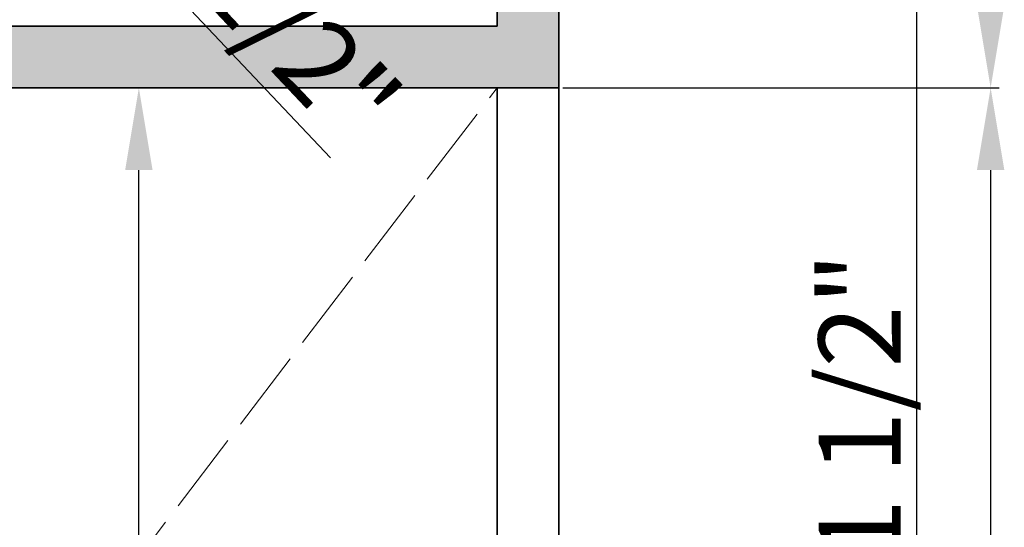
# Model space of a CAD drawing. Units: inches. Extents: x 2083 to 3317, y 1141 to 2115.
# Tile 254 of 256: x 3048 to 3192, y 1639 to 1713. Entities that reach past the tile are written whole.
import ezdxf

# ---------------------------------------------------------------- set-up
doc = ezdxf.new("R2010")
doc.units = ezdxf.units.IN
doc.linetypes.add('ACAD_ISO02W100', pattern=[15, 12, -3])
for name, color, linetype, lineweight in [('A-ANNO-DIMS', 2, 'Continuous', 18), ('A-FLOR-OPEN', 8, 'ACAD_ISO02W100', 13), ('A-WALL', 7, 'Continuous', 35)]:
    doc.layers.add(name, color=color, linetype=linetype, lineweight=lineweight)
doc.layers.add('A-WALL-PATT', color=251, linetype='Continuous', lineweight=13, true_color=0x636466)
doc.styles.get("Standard").update_dxf_attribs({"font": 'arial.ttf'})
doc.dimstyles.new('ISO-25', dxfattribs={"dimtxt": 12, "dimasz": 12, "dimexe": 1.25, "dimexo": 0.625, "dimtad": 1, "dimlunit": 3, "dimtxsty": 'Standard', "dimcen": 2.5, "dimadec": 0, "dimazin": 0, "dimtfac": 1, "dimtmove": 0, "dimatfit": 3, "dimfxl": 1, "dimarcsym": 0})

# ---------------------------------------------------------------- blocks, each defined once
blk = doc.blocks.new('*D7')
at = {"layer": 'A-ANNO-DIMS', "color": 0, "lineweight": -2, "transparency": 16777216}
for p, q in [((3127.58, 2020.76), (3191.32, 2020.76)), ((3190.07, 2008.76), (3190.07, 1714.76)), ((3127.58, 1702.76), (3191.32, 1702.76))]:
    blk.add_line(p, q, dxfattribs=at)
at = {"layer": 'A-ANNO-DIMS', "color": 0, "transparency": 16777216}
for points in [[(3188.07, 2008.76), (3192.07, 2008.76), (3190.07, 2020.76)], [(3188.07, 1714.76), (3192.07, 1714.76), (3190.07, 1702.76)]]:
    blk.add_solid(points, dxfattribs=at)
at = {"layer": 'Defpoints', "color": 0, "transparency": 16777216}
for p in [(3126.96, 2020.76), (3126.96, 1702.76), (3190.07, 1702.76)]:
    blk.add_point(p, dxfattribs=at)
at = {"layer": 'A-ANNO-DIMS', "color": 0, "transparency": 16777216, "insert": (3183.32, 1861.76), "char_height": 12, "attachment_point": 5, "rotation": 90}
blk.add_mtext('26\'-6"', dxfattribs=at)
blk = doc.blocks.new('*D8')
at = {"layer": 'A-ANNO-DIMS', "color": 0, "lineweight": -2, "transparency": 16777216}
for p, q in [((3127.58, 1702.76), (3191.32, 1702.76)), ((3190.07, 1690.76), (3190.07, 1498.76)), ((3127.58, 1486.76), (3191.32, 1486.76))]:
    blk.add_line(p, q, dxfattribs=at)
at = {"layer": 'A-ANNO-DIMS', "color": 0, "transparency": 16777216}
for points in [[(3188.07, 1690.76), (3192.07, 1690.76), (3190.07, 1702.76)], [(3188.07, 1498.76), (3192.07, 1498.76), (3190.07, 1486.76)]]:
    blk.add_solid(points, dxfattribs=at)
at = {"layer": 'Defpoints', "color": 0, "transparency": 16777216}
for p in [(3126.96, 1702.76), (3126.96, 1486.76), (3190.07, 1486.76)]:
    blk.add_point(p, dxfattribs=at)
at = {"layer": 'A-ANNO-DIMS', "color": 0, "transparency": 16777216, "insert": (3183.32, 1594.76), "char_height": 12, "attachment_point": 5, "rotation": 90}
blk.add_mtext("18'", dxfattribs=at)
blk = doc.blocks.new('*D35')
at = {"layer": 'A-ANNO-DIMS', "color": 0, "lineweight": -2, "transparency": 16777216}
for p, q in [((3127.58, 2020.76), (3180.56, 2020.76)), ((3179.31, 1275.26), (3179.31, 2008.76)), ((3127.58, 1263.26), (3180.56, 1263.26))]:
    blk.add_line(p, q, dxfattribs=at)
at = {"layer": 'A-ANNO-DIMS', "color": 0, "transparency": 16777216}
for points in [[(3177.31, 2008.76), (3181.31, 2008.76), (3179.31, 2020.76)], [(3177.31, 1275.26), (3181.31, 1275.26), (3179.31, 1263.26)]]:
    blk.add_solid(points, dxfattribs=at)
at = {"layer": 'Defpoints', "color": 0, "transparency": 16777216}
for p in [(3126.96, 2020.76), (3179.31, 2020.76), (3126.96, 1263.26)]:
    blk.add_point(p, dxfattribs=at)
at = {"layer": 'A-ANNO-DIMS', "color": 0, "transparency": 16777216, "insert": (3172.48, 1642.01), "char_height": 12, "attachment_point": 5, "rotation": 90}
blk.add_mtext('63\'-1 1/2"', dxfattribs=at)
blk = doc.blocks.new('*D65')
at = {"layer": 'A-ANNO-DIMS', "color": 0, "lineweight": -2, "transparency": 16777216}
for p, q in [((3117.33, 1702.76), (3064.36, 1702.76)), ((3065.61, 1498.76), (3065.61, 1690.76)), ((3117.33, 1486.76), (3064.36, 1486.76))]:
    blk.add_line(p, q, dxfattribs=at)
at = {"layer": 'A-ANNO-DIMS', "color": 0, "transparency": 16777216}
for points in [[(3063.61, 1690.76), (3067.61, 1690.76), (3065.61, 1702.76)], [(3063.61, 1498.76), (3067.61, 1498.76), (3065.61, 1486.76)]]:
    blk.add_solid(points, dxfattribs=at)
at = {"layer": 'Defpoints', "color": 0, "transparency": 16777216}
for p in [(3065.61, 1702.76), (3117.96, 1702.76), (3117.96, 1486.76)]:
    blk.add_point(p, dxfattribs=at)
at = {"layer": 'A-ANNO-DIMS', "color": 0, "transparency": 16777216, "insert": (3058.86, 1594.76), "char_height": 12, "attachment_point": 5, "rotation": 90}
blk.add_mtext('18\'-0"', dxfattribs=at)
blk = doc.blocks.new('*D71')
at = {"layer": 'A-ANNO-DIMS', "color": 0, "lineweight": -2, "transparency": 16777216}
for p, q in [((2997.14, 1794.66), (3020.88, 1769.53)), ((3093.61, 1692.52), (3029.12, 1760.8))]:
    blk.add_line(p, q, dxfattribs=at)
at = {"layer": 'A-ANNO-DIMS', "color": 0, "transparency": 16777216}
blk.add_solid([(3030.57, 1762.18), (3027.67, 1759.43), (3020.88, 1769.53)], dxfattribs=at)
at = {"layer": 'Defpoints', "color": 0, "transparency": 16777216}
for p in [(2997.14, 1794.66), (3020.88, 1769.53)]:
    blk.add_point(p, dxfattribs=at)
at = {"layer": 'A-ANNO-DIMS', "color": 0, "transparency": 16777216, "insert": (3070.45, 1726.99), "char_height": 12, "attachment_point": 5, "rotation": 313.3638}
blk.add_mtext('R2\'-10 1/2"', dxfattribs=at)

msp = doc.modelspace()

# ---------------------------------------------------------------- hatches: boundary and pattern name
at = {"layer": 'A-WALL-PATT'}
h = msp.add_hatch(color=256, dxfattribs=at)
h.dxf.hatch_style = 1
h.paths.add_polyline_path([(3126.96, 2020.761), (2748.96, 2020.761), (2604.96, 2020.761), (2226.96, 2020.761), (2226.96, 1702.761), (2466.96, 1702.761), (2466.96, 1582.761), (2418.96, 1582.761), (2418.96, 1477.761), (2226.96, 1477.761), (2226.96, 1263.261), (2544.96, 1263.261), (2544.96, 1411.761), (2604.96, 1411.761), (2685.96, 1411.761), (2685.96, 1420.761), (2604.96, 1420.761), (2604.96, 1573.761), (2604.96, 1702.761), (2604.96, 2011.761), (2748.96, 2011.761), (2748.96, 1702.761), (2862.96, 1702.761), (2862.96, 1621.761), (2871.96, 1621.761), (2871.96, 1702.761), (2883.96, 1702.761), (2883.96, 1706.939, -0.0264593), (2883.96, 1711.761), (2757.96, 1711.761), (2757.96, 1807.761), (2787.96, 1807.761), (2787.96, 1812.261), (2757.96, 1812.261), (2757.96, 2011.761), (2877.96, 2011.761), (2877.96, 1812.261), (2847.96, 1812.261), (2847.96, 1807.761), (2889.836, 1807.761), (2889.836, 1812.261), (2882.46, 1812.261), (2882.46, 2011.761), (3117.96, 2011.761), (3117.96, 1812.261), (2937.836, 1812.261), (2937.836, 1807.761), (2995.71, 1807.761), (2995.71, 1796.118), (3000.21, 1796.118), (3000.21, 1807.761), (3117.96, 1807.761), (3117.96, 1711.761), (3000.21, 1711.761), (3000.21, 1760.118), (2998.573, 1760.118, -0.020711), (2995.71, 1760.118), (2995.71, 1711.761), (2931.96, 1711.761), (2931.96, 1702.761), (3126.96, 1702.761)])
h.paths.add_polyline_path([(2471.46, 2011.761), (2471.46, 1810.011), (2462.717, 1810.011), (2462.717, 1805.511), (2505.96, 1805.511), (2505.96, 1810.011), (2475.96, 1810.011), (2475.96, 2011.761), (2595.96, 2011.761), (2595.96, 1810.011), (2565.96, 1810.011), (2565.96, 1805.511), (2595.96, 1805.511), (2595.96, 1711.761), (2235.96, 1711.761), (2235.96, 1805.511), (2353.71, 1805.511), (2353.71, 1796.054), (2358.21, 1796.054), (2358.21, 1805.511), (2414.717, 1805.511), (2414.717, 1810.011), (2235.96, 1810.011), (2235.96, 2011.761)], flags=16)
h.paths.add_polyline_path([(2270.205, 1994.61), (2270.205, 1970.61), (2246.205, 1970.61), (2246.205, 1994.61)], flags=0)
edge = h.paths.add_edge_path(flags=0)
edge.add_ellipse((2332.027, 1899.798), major_axis=(-3.043, 3.043), ratio=0.1682525, start_angle=-161.33217, end_angle=-156.30711, ccw=False)
edge.add_ellipse((2333.082, 1898.744), major_axis=(-1.055, 1.055), ratio=0.4535321, start_angle=-123.37102, end_angle=-94.15911)
edge = h.paths.add_edge_path(flags=0)
edge.add_ellipse((2332.027, 1968.876), major_axis=(3.043, 3.043), ratio=0.1682525, start_angle=18.66783, end_angle=23.69289)
edge.add_spline(control_points=[(2332.926, 1970.691), (2332.227, 1970.336), (2330.894, 1969.659), (2328.413, 1970.932), (2327.204, 1967.749), (2324.71, 1969.956), (2322.533, 1967.012), (2320.013, 1971.296), (2317.68, 1968.158), (2316.041, 1967.102), (2315.427, 1966.81)], knot_values=[0, 0, 0, 0, 2.2670587, 4.3245589, 6.6855835, 8.8786411, 11.121502, 14.300359, 17.7552837, 19.732645, 19.732645, 19.732645, 19.732645], degree=3, periodic=0)
edge.add_ellipse((2332.027, 1968.876), major_axis=(3.043, 3.043), ratio=0.1682525, start_angle=18.66783, end_angle=23.69289, ccw=False)
edge.add_ellipse((2333.082, 1969.931), major_axis=(1.055, 1.055), ratio=0.4535321, start_angle=56.62898, end_angle=85.84089, ccw=False)
edge = h.paths.add_edge_path(flags=0)
edge.add_spline(control_points=[(2296.428, 1967.988), (2293.628, 1965.336), (2287.704, 1959.727), (2299.744, 1949.996), (2294.533, 1935.669), (2290.573, 1920.604), (2293.394, 1909.974), (2296.185, 1904.967)], knot_values=[0.0991853, 0.0991853, 0.0991853, 0.0991853, 0.3453009, 0.6198217, 0.9826526, 1.3860932, 1.8105546, 1.8105546, 1.8105546, 1.8105546], degree=3, periodic=0)
edge.add_spline(control_points=[(2296.185, 1904.967), (2297.384, 1902.619), (2298.001, 1901.949), (2298.553, 1901.468)], knot_values=[0.0062457, 0.0062457, 0.0062457, 0.0062457, 0.0554759, 0.0554759, 0.0554759, 0.0554759], degree=3, periodic=0)
edge.add_spline(control_points=[(2298.553, 1901.468), (2297.259, 1900.923), (2295.225, 1900.232), (2293.06, 1900.614), (2292.101, 1900.788), (2292.09, 1900.791)], knot_values=[0.3128349, 0.3128349, 0.3128349, 0.3128349, 0.4017797, 0.4749867, 0.4759027, 0.4759027, 0.4759027, 0.4759027], degree=3, periodic=0)
edge.add_arc((2292.794, 1904.664), 3.937, 215.4209, 259.69818, ccw=False)
edge.add_spline(control_points=[(2289.585, 1902.382), (2289.477, 1902.535), (2289.368, 1902.688), (2289.261, 1902.841)], knot_values=[0.1028719, 0.1028719, 0.1028719, 0.1028719, 0.1168958, 0.1168958, 0.1168958, 0.1168958], degree=3, periodic=0)
edge.add_spline(control_points=[(2289.261, 1902.841), (2288.687, 1902.55), (2287.64, 1902.02), (2285.881, 1901.874), (2283.853, 1901.504), (2281.72, 1899.711), (2278.467, 1899.493), (2276.157, 1901.883), (2272.259, 1899.804), (2267.778, 1901.843), (2262.244, 1900.184), (2257.415, 1901.782), (2254.318, 1900.726), (2253.178, 1900.337)], knot_values=[0, 0, 0, 0, 1.9079767, 3.4771759, 5.261074, 7.9728515, 11.6802485, 13.7179214, 16.9395917, 22.789562, 27.5025027, 33.5952153, 37.1456181, 37.1456181, 37.1456181, 37.1456181], degree=3, periodic=0)
edge.add_line((2253.178, 1900.337), (2250.244, 1902.841))
edge.add_line((2250.244, 1902.841), (2250.244, 1965.833))
edge.add_line((2250.244, 1965.833), (2253.178, 1968.337))
edge.add_spline(control_points=[(2253.178, 1968.337), (2254.318, 1967.948), (2257.415, 1966.892), (2262.244, 1968.49), (2267.778, 1966.831), (2271.527, 1968.537), (2273.876, 1967.828), (2274.207, 1967.728)], knot_values=[0, 0, 0, 0, 0.0901802, 0.2449351, 0.3646438, 0.5132331, 0.5378548, 0.5378548, 0.5378548, 0.5378548], degree=3, periodic=0)
edge.add_arc((2274.353, 1963.793), 3.937, 72.05113, 92.12795, ccw=False)
edge.add_arc((2281.297, 1985.23), 18.596, 252.05113, 288.56572)
edge.add_arc((2292.317, 1956.029), 12.646, 71.02679, 113.77822, ccw=False)
edge = h.paths.add_edge_path(flags=0)
edge.add_spline(control_points=[(2274.899, 1951.856), (2275.066, 1951.617), (2275.233, 1951.377), (2275.398, 1951.136)], knot_values=[1.4099157, 1.4099157, 1.4099157, 1.4099157, 1.4315903, 1.4315903, 1.4315903, 1.4315903], degree=3, periodic=0)
edge.add_spline(control_points=[(2275.398, 1951.136), (2275.792, 1950.562), (2276.179, 1949.984), (2276.546, 1949.397)], knot_values=[1.3582378, 1.3582378, 1.3582378, 1.3582378, 1.4099157, 1.4099157, 1.4099157, 1.4099157], degree=3, periodic=0)
edge.add_line((2276.546, 1949.397), (2277.437, 1947.862))
edge.add_spline(control_points=[(2277.437, 1947.862), (2276.304, 1945.673), (2274.64, 1942.427), (2274.632, 1938.094), (2272.799, 1930.852), (2274.356, 1943.897), (2275.948, 1947.923), (2276.546, 1949.397)], knot_values=[0.0056315, 0.0056315, 0.0056315, 0.0056315, 0.1860139, 0.2660015, 0.3570872, 0.5963902, 0.7397317, 0.7397317, 0.7397317, 0.7397317], degree=3, periodic=0)
edge.add_spline(control_points=[(2276.546, 1949.397), (2276.179, 1949.984), (2275.792, 1950.562), (2275.398, 1951.136)], knot_values=[1.3582378, 1.3582378, 1.3582378, 1.3582378, 1.4099157, 1.4099157, 1.4099157, 1.4099157], degree=3, periodic=0)
edge.add_spline(control_points=[(2275.398, 1951.136), (2274.943, 1950.08), (2274.208, 1948.025), (2273.935, 1944.851), (2272.469, 1937.627), (2273.466, 1945.696), (2274.701, 1951.059), (2274.899, 1951.856)], knot_values=[0.1043639, 0.1043639, 0.1043639, 0.1043639, 0.1896363, 0.2696239, 0.3607096, 0.6000126, 0.6446217, 0.6446217, 0.6446217, 0.6446217], degree=3, periodic=0)
h.paths.add_polyline_path([(2269.168, 1963.128, -0.3575267), (2268.171, 1960.976, -0.0925607), (2268.171, 1939.436, -0.3575267), (2269.168, 1937.285, -0.3575267), (2267.016, 1938.282, -0.1647847), (2254.686, 1938.282, -0.3575267), (2252.534, 1937.285, -0.3575267), (2253.531, 1939.436, -0.0925607), (2253.531, 1960.976, -0.3575267), (2252.534, 1963.128, -0.3575267), (2254.686, 1962.131, -0.1647847), (2267.016, 1962.131, -0.3575267)], flags=0)
h.paths.add_polyline_path([(2248.874, 1967.802), (2248.874, 1957.028), (2249.458, 1957.028), (2249.458, 1911.647), (2248.874, 1911.647), (2248.874, 1900.873), (2246.512, 1900.873, 0.1973271), (2244.15, 1902.457), (2244.15, 1966.218, 0.1973271), (2246.512, 1967.802)], flags=0)
h.paths.add_polyline_path([(2269.168, 1931.389, -0.3575267), (2268.171, 1929.238, -0.0925607), (2268.171, 1907.698, -0.3575267), (2269.168, 1905.547, -0.3575267), (2267.016, 1906.544, -0.1647847), (2254.686, 1906.544, -0.3575267), (2252.534, 1905.547, -0.3575267), (2253.531, 1907.698, -0.0925607), (2253.531, 1929.238, -0.3575267), (2252.534, 1931.389, -0.3575267), (2254.686, 1930.392, -0.1647847), (2267.016, 1930.392, -0.3575267)], flags=0)
edge = h.paths.add_edge_path(flags=0)
edge.add_spline(control_points=[(2276.197, 1906.724), (2276.168, 1909.029), (2276.114, 1913.372), (2270.598, 1924.925), (2273.905, 1919.013), (2275.922, 1916.262), (2275.475, 1912.402), (2277.258, 1910.381), (2276.696, 1908.225), (2276.646, 1906.813), (2276.618, 1906.008)], knot_values=[0, 0, 0, 0, 8.6102597, 16.2212739, 18.8430575, 23.8048978, 27.4408283, 29.3561016, 31.2034776, 33.6506866, 33.6506866, 33.6506866, 33.6506866], degree=3, periodic=0)
edge.add_spline(control_points=[(2276.618, 1906.008), (2276.623, 1905.624), (2276.498, 1904.629), (2275.442, 1903.855), (2274.937, 1903.08), (2274.859, 1902.841)], knot_values=[0.1564884, 0.1564884, 0.1564884, 0.1564884, 0.1843975, 0.2313765, 0.2505985, 0.2505985, 0.2505985, 0.2505985], degree=3, periodic=0)
edge.add_line((2274.859, 1902.841), (2276.506, 1902.841))
edge.add_spline(control_points=[(2276.506, 1902.841), (2276.788, 1903.085), (2277.665, 1904.125), (2278.25, 1904.341), (2277.654, 1908.527), (2278.156, 1906.228), (2278.1, 1905.286), (2278.847, 1904.069), (2277.857, 1903.415), (2277.874, 1902.991), (2277.904, 1902.841)], knot_values=[0.0595743, 0.0595743, 0.0595743, 0.0595743, 0.0807529, 0.1037415, 0.1697201, 0.1760361, 0.2071372, 0.2404744, 0.2623409, 0.2736605, 0.2736605, 0.2736605, 0.2736605], degree=3, periodic=0)
edge.add_line((2277.904, 1902.841), (2280.03, 1902.841))
edge.add_spline(control_points=[(2280.03, 1902.841), (2279.888, 1903.088), (2279.499, 1903.982), (2280.152, 1905.939), (2278.104, 1909.658), (2279.762, 1907.185), (2280.328, 1904.875), (2280.485, 1903.49), (2281.463, 1903.249), (2281.758, 1902.936), (2281.834, 1902.841)], knot_values=[0.013856, 0.013856, 0.013856, 0.013856, 0.0348738, 0.0888667, 0.1078792, 0.1267378, 0.158714, 0.1937575, 0.2174868, 0.2267221, 0.2267221, 0.2267221, 0.2267221], degree=3, periodic=0)
edge.add_spline(control_points=[(2281.834, 1902.841), (2281.788, 1902.827), (2281.647, 1902.783), (2281.396, 1902.859), (2281.088, 1902.985), (2280.721, 1903.061), (2280.333, 1903.026), (2280.125, 1902.899), (2280.03, 1902.841)], knot_values=[0, 0, 0, 0, 0.1441304, 0.435517, 0.7492759, 1.1530457, 1.5483707, 1.878348, 1.878348, 1.878348, 1.878348], degree=3, periodic=0)
edge.add_line((2280.03, 1902.841), (2277.904, 1902.841))
edge.add_spline(control_points=[(2277.904, 1902.841), (2277.893, 1902.796), (2277.865, 1902.68), (2277.607, 1902.687), (2277.274, 1902.801), (2276.838, 1902.62), (2276.584, 1902.789), (2276.506, 1902.841)], knot_values=[0, 0, 0, 0, 0.1271885, 0.3261988, 0.6280094, 1.2435704, 1.5153306, 1.5153306, 1.5153306, 1.5153306], degree=3, periodic=0)
edge.add_line((2276.506, 1902.841), (2274.859, 1902.841))
edge.add_spline(control_points=[(2274.859, 1902.841), (2274.814, 1902.899), (2274.725, 1903.013), (2274.493, 1903.119), (2274.244, 1902.961), (2273.937, 1903.185), (2273.614, 1902.983), (2273.408, 1902.883), (2273.322, 1902.841)], knot_values=[0, 0, 0, 0, 0.2184302, 0.4369566, 0.6879766, 0.9903786, 1.3983955, 1.6918498, 1.6918498, 1.6918498, 1.6918498], degree=3, periodic=0)
edge.add_spline(control_points=[(2273.322, 1902.841), (2273.617, 1903.446), (2274.274, 1904.538), (2276.027, 1904.574), (2276.207, 1906.584), (2276.197, 1906.724)], knot_values=[0.0122268, 0.0122268, 0.0122268, 0.0122268, 0.0594721, 0.1062177, 0.134458, 0.134458, 0.134458, 0.134458], degree=3, periodic=0)
h.paths.add_polyline_path([(2270.776, 1897.79), (2270.776, 1873.79), (2246.776, 1873.79), (2246.776, 1897.79)], flags=0)
h.paths.add_polyline_path([(2353.71, 1760.005), (2353.71, 1760.054), (2358.21, 1760.054, -0.033729)], flags=0)
h.paths.add_polyline_path([(2321.819, 1737.529), (2341.995, 1737.529, -0.4142136), (2343.203, 1736.321), (2343.203, 1721.021, -0.4142136), (2341.995, 1719.813), (2321.819, 1719.813, -0.4142136), (2320.611, 1721.021), (2320.611, 1736.321, -0.4142136)], flags=0)
h.paths.add_polyline_path([(2324.235, 1736.321), (2339.579, 1736.321, -0.4142136), (2341.995, 1733.905), (2341.995, 1725.45, -0.4142136), (2339.579, 1723.034), (2333.681, 1723.034), (2333.845, 1722.045, -0.8706461), (2335.425, 1721.826, -0.767327), (2333.923, 1721.423), (2331.291, 1721.423, -0.767327), (2329.788, 1721.826, -0.8706461), (2331.368, 1722.045), (2331.533, 1723.034), (2324.235, 1723.034, -0.4142136), (2321.819, 1725.45), (2321.819, 1733.905, -0.4142136)], flags=0)
h.paths.add_polyline_path([(2570.484, 1928.615), (2589.684, 1928.615), (2590.169, 1928.615), (2590.169, 1904.993), (2570.484, 1904.993)], flags=0)
h.paths.add_polyline_path([(2574.447, 1927.264, -1), (2572.829, 1927.264, -1)], flags=0)
h.paths.add_polyline_path([(2573.09, 1926.941), (2573.925, 1927.776), (2574.148, 1927.553), (2573.313, 1926.718)], flags=0)
h.paths.add_polyline_path([(2578.779, 1919.73, -1), (2571.592, 1919.73, -1)], flags=0)
h.paths.add_polyline_path([(2578.385, 1919.73, -1), (2571.985, 1919.73, -1)], flags=0)
h.paths.add_polyline_path([(2331.596, 1729.476, -1), (2333.618, 1729.476, -1)], flags=0)
h.paths.add_polyline_path([(2578.034, 1927.264, -1), (2576.416, 1927.264, -1)], flags=0)
h.paths.add_polyline_path([(2576.689, 1927.531), (2576.912, 1927.754), (2577.747, 1926.919), (2577.524, 1926.696)], flags=0)
h.paths.add_polyline_path([(2578.139, 1909.86, -1), (2572.232, 1909.86, -1)], flags=0)
h.paths.add_polyline_path([(2577.745, 1909.86, -1), (2572.625, 1909.86, -1)], flags=0)
h.paths.add_polyline_path([(2583.798, 1927.264, -1), (2582.179, 1927.264, -1)], flags=0)
h.paths.add_polyline_path([(2582.719, 1927.754), (2583.554, 1926.919), (2583.331, 1926.696), (2582.496, 1927.531)], flags=0)
h.paths.add_polyline_path([(2582.496, 1927.531), (2582.719, 1927.754), (2583.554, 1926.919), (2583.331, 1926.696)], flags=0)
h.paths.add_polyline_path([(2587.739, 1920.53, -1), (2581.832, 1920.53, -1)], flags=0)
h.paths.add_polyline_path([(2587.345, 1920.53, -1), (2582.225, 1920.53, -1)], flags=0)
h.paths.add_polyline_path([(2587.385, 1927.264, -1), (2585.766, 1927.264, -1)], flags=0)
h.paths.add_polyline_path([(2586.082, 1926.98), (2586.917, 1927.815), (2587.14, 1927.593), (2586.305, 1926.758)], flags=0)
h.paths.add_polyline_path([(2588.379, 1910.66, -1), (2581.192, 1910.66, -1)], flags=0)
h.paths.add_polyline_path([(2587.985, 1910.66, -1), (2581.585, 1910.66, -1)], flags=0)
h.paths.add_polyline_path([(2417.168, 1729.478), (2437.344, 1729.478, -0.4142136), (2438.552, 1728.27), (2438.552, 1712.969, -0.4142136), (2437.344, 1711.761), (2417.168, 1711.761, -0.4142136), (2415.96, 1712.969), (2415.96, 1728.27, -0.4142136)], flags=0)
h.paths.add_polyline_path([(2419.584, 1728.27), (2434.928, 1728.27, -0.4142136), (2437.344, 1725.854), (2437.344, 1717.398, -0.4142136), (2434.928, 1714.983), (2429.029, 1714.983), (2429.194, 1713.994, -0.8706461), (2430.774, 1713.775, -0.767327), (2429.271, 1713.372), (2426.64, 1713.372, -0.767327), (2425.137, 1713.775, -0.8706461), (2426.717, 1713.994), (2426.882, 1714.983), (2419.584, 1714.983, -0.4142136), (2417.168, 1717.398), (2417.168, 1725.854, -0.4142136)], flags=0)
h.paths.add_polyline_path([(2419.584, 1728.27), (2434.928, 1728.27, -0.4142136), (2437.344, 1725.854), (2437.344, 1717.398, -0.4142136), (2434.928, 1714.983), (2429.029, 1714.983), (2428.358, 1719.009), (2427.553, 1719.009), (2426.882, 1714.983), (2419.584, 1714.983, -0.4142136), (2417.168, 1717.398), (2417.168, 1725.854, -0.4142136)], flags=0)
h.paths.add_polyline_path([(2426.944, 1721.425, -1), (2428.967, 1721.425, -1)], flags=0)
h.paths.add_polyline_path([(2475.96, 1702.761), (2595.96, 1702.761), (2595.96, 1582.761), (2475.96, 1582.761)], flags=16)
h.paths.add_polyline_path([(2427.96, 1573.761), (2595.96, 1573.761), (2595.96, 1468.761), (2595.96, 1420.761), (2384.46, 1420.761), (2384.46, 1468.761), (2427.96, 1468.761)], flags=16)
h.paths.add_polyline_path([(2379.96, 1468.761), (2379.96, 1420.761), (2235.96, 1420.761), (2235.96, 1468.761)], flags=16)
h.paths.add_polyline_path([(2317.816, 1466.696), (2337.992, 1466.696, -0.4142136), (2339.2, 1465.488), (2339.2, 1450.187, -0.4142136), (2337.992, 1448.979), (2317.816, 1448.979, -0.4142136), (2316.608, 1450.187), (2316.608, 1465.488, -0.4142136)], flags=0)
h.paths.add_polyline_path([(2320.232, 1465.488), (2335.576, 1465.488, -0.4142136), (2337.992, 1463.072), (2337.992, 1454.616, -0.4142136), (2335.576, 1452.2), (2329.677, 1452.2), (2329.842, 1451.212, -0.8706461), (2331.422, 1450.992, -0.767327), (2329.92, 1450.59), (2327.288, 1450.59, -0.767327), (2325.785, 1450.992, -0.8706461), (2327.365, 1451.212), (2327.53, 1452.2), (2320.232, 1452.2, -0.4142136), (2317.816, 1454.616), (2317.816, 1463.072, -0.4142136)], flags=0)
h.paths.add_polyline_path([(2320.232, 1465.488), (2335.576, 1465.488, -0.4142136), (2337.992, 1463.072), (2337.992, 1454.616, -0.4142136), (2335.576, 1452.2), (2329.677, 1452.2), (2329.006, 1456.227), (2328.201, 1456.227), (2327.53, 1452.2), (2320.232, 1452.2, -0.4142136), (2317.816, 1454.616), (2317.816, 1463.072, -0.4142136)], flags=0)
h.paths.add_polyline_path([(2327.593, 1458.643, -1), (2329.615, 1458.643, -1)], flags=0)
h.paths.add_polyline_path([(2244.412, 1433.34), (2241.921, 1433.34, -0.4142136), (2240.018, 1435.244), (2240.018, 1440.953, -0.4142105), (2241.921, 1442.856), (2244.412, 1442.856, -1.9764724)], flags=0)
h.paths.add_polyline_path([(2245.357, 1434.398, -0.4142136), (2245.357, 1441.799, -2.1440985)], flags=0)
h.paths.add_polyline_path([(2535.96, 1416.261), (2535.96, 1272.261), (2235.96, 1272.261), (2235.96, 1416.261)], flags=16)
h.paths.add_polyline_path([(2260.12, 1384.293), (2260.12, 1362.039), (2237.865, 1362.039), (2237.865, 1384.293)], flags=0)
edge = h.paths.add_edge_path(flags=0)
edge.add_line((2318.252, 1362.093), (2318.146, 1362.001))
edge.add_ellipse((2317.445, 1360.431), major_axis=(2.822, 2.822), ratio=0.1682525, start_angle=18.66783, end_angle=20.94813, ccw=False)
edge.add_ellipse((2318.423, 1361.409), major_axis=(0.978, 0.978), ratio=0.4535321, start_angle=56.62898, end_angle=70.2262, ccw=False)
edge = h.paths.add_edge_path(flags=0)
edge.add_line((2319.107, 1295.571), (2319.015, 1295.677))
edge.add_ellipse((2317.445, 1296.378), major_axis=(-2.822, 2.822), ratio=0.1682525, start_angle=-161.33217, end_angle=-159.05187, ccw=False)
edge.add_ellipse((2318.423, 1295.4), major_axis=(-0.978, 0.978), ratio=0.4535321, start_angle=-123.37102, end_angle=-109.7738)
edge = h.paths.add_edge_path(flags=0)
edge.add_spline(control_points=[(2284.21, 1301.17), (2284.581, 1300.445), (2284.891, 1299.892), (2285.16, 1299.461)], knot_values=[0.0390658, 0.0390658, 0.0390658, 0.0390658, 0.0554759, 0.0554759, 0.0554759, 0.0554759], degree=3, periodic=0)
edge.add_line((2285.16, 1299.461), (2284.21, 1301.17))
edge = h.paths.add_edge_path(flags=0)
edge.add_line((2280.412, 1297.298), (2283.37, 1297.036))
edge.add_line((2283.37, 1297.036), (2286.406, 1297.926))
edge.add_spline(control_points=[(2286.406, 1297.926), (2285.305, 1297.463), (2284.345, 1297.129), (2283.37, 1297.036)], knot_values=[0.3943688, 0.3943688, 0.3943688, 0.3943688, 0.4759027, 0.4759027, 0.4759027, 0.4759027], degree=3, periodic=0)
edge.add_spline(control_points=[(2283.37, 1297.036), (2283.281, 1297.028), (2282.316, 1296.957), (2281.313, 1297.134), (2280.423, 1297.296), (2280.412, 1297.298)], knot_values=[0.3128349, 0.3128349, 0.3128349, 0.3128349, 0.3202458, 0.3934528, 0.3943688, 0.3943688, 0.3943688, 0.3943688], degree=3, periodic=0)
edge = h.paths.add_edge_path(flags=0)
edge.add_line((2284.436, 1359.607), (2280.446, 1355.328))
edge.add_line((2280.446, 1355.328), (2279.58, 1351.018))
edge.add_line((2279.58, 1351.018), (2282.413, 1346.58))
edge.add_spline(control_points=[(2282.413, 1346.58), (2283.153, 1345.589), (2284.253, 1344.029), (2284.801, 1342.387), (2284.935, 1341.806)], knot_values=[1.2400982, 1.2400982, 1.2400982, 1.2400982, 1.3328922, 1.3827123, 1.3827123, 1.3827123, 1.3827123], degree=3, periodic=0)
edge.add_spline(control_points=[(2284.935, 1341.806), (2285.319, 1340.141), (2285.233, 1338.409), (2284.91, 1336.654)], knot_values=[1.0974841, 1.0974841, 1.0974841, 1.0974841, 1.2400982, 1.2400982, 1.2400982, 1.2400982], degree=3, periodic=0)
edge.add_spline(control_points=[(2284.91, 1336.654), (2284.587, 1334.899), (2284.027, 1333.12), (2283.463, 1331.361)], knot_values=[0.9548699, 0.9548699, 0.9548699, 0.9548699, 1.0974841, 1.0974841, 1.0974841, 1.0974841], degree=3, periodic=0)
edge.add_line((2283.463, 1331.361), (2281.89, 1326.153))
edge.add_line((2281.89, 1326.153), (2280.756, 1321.056))
edge.add_line((2280.756, 1321.056), (2280.299, 1316.002))
edge.add_line((2280.299, 1316.002), (2280.716, 1310.95))
edge.add_line((2280.716, 1310.95), (2282.028, 1305.972))
edge.add_line((2282.028, 1305.972), (2284.21, 1301.17))
edge.add_spline(control_points=[(2284.21, 1301.17), (2283.341, 1302.73), (2282.612, 1304.336), (2282.028, 1305.972)], knot_values=[0.0991853, 0.0991853, 0.0991853, 0.0991853, 0.2417994, 0.2417994, 0.2417994, 0.2417994], degree=3, periodic=0)
edge.add_spline(control_points=[(2282.028, 1305.972), (2281.444, 1307.608), (2281.005, 1309.273), (2280.716, 1310.95)], knot_values=[0.2417994, 0.2417994, 0.2417994, 0.2417994, 0.3844135, 0.3844135, 0.3844135, 0.3844135], degree=3, periodic=0)
edge.add_spline(control_points=[(2280.716, 1310.95), (2280.433, 1312.588), (2280.289, 1314.277), (2280.299, 1315.962), (2280.299, 1316.002)], knot_values=[0.3844135, 0.3844135, 0.3844135, 0.3844135, 0.5236467, 0.5270276, 0.5270276, 0.5270276, 0.5270276], degree=3, periodic=0)
edge.add_spline(control_points=[(2280.299, 1316.002), (2280.312, 1317.687), (2280.478, 1319.368), (2280.756, 1321.056)], knot_values=[0.5270276, 0.5270276, 0.5270276, 0.5270276, 0.6696417, 0.6696417, 0.6696417, 0.6696417], degree=3, periodic=0)
edge.add_spline(control_points=[(2280.756, 1321.056), (2281.035, 1322.744), (2281.426, 1324.44), (2281.89, 1326.153)], knot_values=[0.6696417, 0.6696417, 0.6696417, 0.6696417, 0.8122558, 0.8122558, 0.8122558, 0.8122558], degree=3, periodic=0)
edge.add_spline(control_points=[(2281.89, 1326.153), (2282.264, 1327.533), (2282.788, 1329.262), (2283.353, 1331.018), (2283.463, 1331.361)], knot_values=[0.8122558, 0.8122558, 0.8122558, 0.8122558, 0.9270873, 0.9548699, 0.9548699, 0.9548699, 0.9548699], degree=3, periodic=0)
edge.add_line((2283.463, 1331.361), (2284.91, 1336.654))
edge.add_line((2284.91, 1336.654), (2284.935, 1341.806))
edge.add_line((2284.935, 1341.806), (2282.413, 1346.58))
edge.add_spline(control_points=[(2282.413, 1346.58), (2281.275, 1348.104), (2280.078, 1349.57), (2279.58, 1351.018)], knot_values=[1.3827123, 1.3827123, 1.3827123, 1.3827123, 1.5253264, 1.5253264, 1.5253264, 1.5253264], degree=3, periodic=0)
edge.add_spline(control_points=[(2279.58, 1351.018), (2279.443, 1351.415), (2279.136, 1352.857), (2279.735, 1354.29), (2280.446, 1355.328)], knot_values=[1.5253264, 1.5253264, 1.5253264, 1.5253264, 1.564439, 1.6679405, 1.6679405, 1.6679405, 1.6679405], degree=3, periodic=0)
edge.add_spline(control_points=[(2280.446, 1355.328), (2281.426, 1356.758), (2282.931, 1358.183), (2284.436, 1359.607)], knot_values=[1.6679405, 1.6679405, 1.6679405, 1.6679405, 1.8105546, 1.8105546, 1.8105546, 1.8105546], degree=3, periodic=0)
edge.add_arc((2280.623, 1348.518), 11.726, 71.02679, 113.77822)
edge.add_arc((2270.405, 1375.595), 17.244, 252.05113, 288.56572, ccw=False)
edge.add_arc((2263.966, 1355.718), 3.651, 72.05113, 92.12795)
edge.add_arc((2263.966, 1355.718), 3.651, 92.12795, 177.98513)
edge.add_spline(control_points=[(2260.318, 1355.846), (2260.26, 1354.221), (2260.551, 1350.187), (2262.999, 1346.766), (2264.473, 1344.649)], knot_values=[1.4315903, 1.4315903, 1.4315903, 1.4315903, 1.5641438, 1.7706953, 1.7706953, 1.7706953, 1.7706953], degree=3, periodic=0)
edge.add_line((2264.473, 1344.649), (2264.936, 1343.983))
edge.add_spline(control_points=[(2263.801, 1340.248), (2263.843, 1340.514), (2264.067, 1341.756), (2264.513, 1343.002), (2264.935, 1343.981)], knot_values=[0.5365702, 0.5365702, 0.5365702, 0.5365702, 0.5593494, 0.6446217, 0.6446217, 0.6446217, 0.6446217], degree=3, periodic=0)
edge.add_spline(control_points=[(2264.935, 1343.981), (2265.118, 1343.715), (2265.299, 1343.448), (2265.477, 1343.179)], knot_values=[1.3840767, 1.3840767, 1.3840767, 1.3840767, 1.4099157, 1.4099157, 1.4099157, 1.4099157], degree=3, periodic=0)
edge.add_spline(control_points=[(2265.477, 1343.179), (2265.655, 1342.911), (2265.829, 1342.641), (2265.999, 1342.369)], knot_values=[1.3582378, 1.3582378, 1.3582378, 1.3582378, 1.3840767, 1.3840767, 1.3840767, 1.3840767], degree=3, periodic=0)
edge.add_line((2265.999, 1342.369), (2266.826, 1340.946))
edge.add_spline(control_points=[(2266.826, 1340.946), (2268.894, 1337.09), (2271.398, 1325.843), (2270.516, 1310.569), (2275.919, 1301.861), (2277.79, 1299.199)], knot_values=[0.1168958, 0.1168958, 0.1168958, 0.1168958, 0.4729873, 1.0509689, 1.3137934, 1.3137934, 1.3137934, 1.3137934], degree=3, periodic=0)
edge.add_spline(control_points=[(2277.79, 1299.199), (2277.839, 1299.128), (2277.889, 1299.057), (2277.94, 1298.987)], knot_values=[0.1098839, 0.1098839, 0.1098839, 0.1098839, 0.1168958, 0.1168958, 0.1168958, 0.1168958], degree=3, periodic=0)
edge.add_line((2277.94, 1298.987), (2277.789, 1299.199))
edge.add_spline(control_points=[(2277.789, 1299.199), (2277.257, 1298.929), (2276.286, 1298.438), (2275.039, 1298.334), (2274.383, 1298.239), (2274.215, 1298.209)], knot_values=[33.1218702, 33.1218702, 33.1218702, 33.1218702, 35.0290557, 36.5982549, 37.1448269, 37.1448269, 37.1448269, 37.1448269], degree=3, periodic=0)
edge.add_line((2274.215, 1298.209), (2273.073, 1297.893))
edge.add_spline(control_points=[(2273.073, 1297.893), (2272.323, 1297.58), (2271.039, 1296.511), (2269.248, 1296.226), (2268.423, 1296.375)], knot_values=[26.5325843, 26.5325843, 26.5325843, 26.5325843, 29.198919, 31.8391012, 31.8391012, 31.8391012, 31.8391012], degree=3, periodic=0)
edge.add_line((2268.423, 1296.375), (2263.879, 1297.458))
edge.add_spline(control_points=[(2263.879, 1297.458), (2263.556, 1297.359), (2261.86, 1296.839), (2260.239, 1297.282), (2258.933, 1297.516)], knot_values=[15.9195506, 15.9195506, 15.9195506, 15.9195506, 16.9395917, 21.2260675, 21.2260675, 21.2260675, 21.2260675], degree=3, periodic=0)
edge.add_line((2258.933, 1297.516), (2254.055, 1297.329))
edge.add_spline(control_points=[(2254.055, 1297.329), (2253.756, 1297.296), (2252.114, 1297.165), (2250.462, 1297.544), (2249.13, 1297.668)], knot_values=[5.3065169, 5.3065169, 5.3065169, 5.3065169, 6.2764352, 10.6130337, 10.6130337, 10.6130337, 10.6130337], degree=3, periodic=0)
edge.add_line((2249.13, 1297.668), (2244.332, 1296.878))
edge.add_line((2244.332, 1296.878), (2241.611, 1299.199))
edge.add_line((2241.611, 1299.199), (2241.611, 1357.609))
edge.add_line((2241.611, 1357.609), (2244.332, 1359.931))
edge.add_line((2244.332, 1359.931), (2252.729, 1359.543))
edge.add_spline(control_points=[(2252.729, 1359.543), (2252.871, 1359.546), (2253.306, 1359.548), (2253.74, 1359.514), (2254.032, 1359.482)], knot_values=[0.233291, 0.233291, 0.233291, 0.233291, 0.2449351, 0.2689274, 0.2689274, 0.2689274, 0.2689274], degree=3, periodic=0)
edge.add_line((2254.032, 1359.482), (2259.587, 1359.416))
edge.add_spline(control_points=[(2259.587, 1359.416), (2260.677, 1359.629), (2262.073, 1359.897), (2263.524, 1359.459), (2263.83, 1359.366)], knot_values=[0.4225164, 0.4225164, 0.4225164, 0.4225164, 0.5132331, 0.5378548, 0.5378548, 0.5378548, 0.5378548], degree=3, periodic=0)
edge.add_arc((2263.966, 1355.718), 3.651, 72.05113, 92.12795, ccw=False)
edge.add_arc((2270.405, 1375.595), 17.244, 252.05113, 288.56572)
edge.add_arc((2280.623, 1348.518), 11.726, 71.02679, 113.77822, ccw=False)
h.paths.add_polyline_path([(2240.341, 1359.435), (2240.341, 1349.444), (2240.882, 1349.444), (2240.882, 1307.365), (2240.341, 1307.365), (2240.341, 1297.374), (2238.15, 1297.374, 0.1973271), (2235.96, 1298.843), (2235.96, 1357.966, 0.1973271), (2238.15, 1359.435)], flags=0)
h.paths.add_polyline_path([(2259.158, 1355.101, -0.3575267), (2258.233, 1353.106, -0.0925607), (2258.233, 1333.133, -0.3575267), (2259.158, 1331.138, -0.3575267), (2257.163, 1332.062, -0.1647847), (2245.729, 1332.062, -0.3575267), (2243.735, 1331.138, -0.3575267), (2244.659, 1333.133, -0.0925607), (2244.659, 1353.106, -0.3575267), (2243.735, 1355.101, -0.3575267), (2245.729, 1354.176, -0.1647847), (2257.163, 1354.176, -0.3575267)], flags=0)
edge = h.paths.add_edge_path(flags=0)
edge.add_line((2265.999, 1342.369), (2266.826, 1340.946))
edge.add_line((2266.826, 1340.946), (2265.308, 1337.814))
edge.add_line((2265.308, 1337.814), (2264.358, 1334.653))
edge.add_line((2264.358, 1334.653), (2264.262, 1333.8))
edge.add_spline(control_points=[(2264.262, 1333.8), (2264.208, 1333.187), (2264.162, 1332.366), (2264.007, 1331.414), (2263.969, 1331.202)], knot_values=[0.4644442, 0.4644442, 0.4644442, 0.4644442, 0.5166905, 0.5316081, 0.5316081, 0.5316081, 0.5316081], degree=3, periodic=0)
edge.add_spline(control_points=[(2263.969, 1331.202), (2263.775, 1330.119), (2263.424, 1328.791), (2263.257, 1328.531), (2263.234, 1328.515)], knot_values=[0.3726816, 0.3726816, 0.3726816, 0.3726816, 0.4488497, 0.4644442, 0.4644442, 0.4644442, 0.4644442], degree=3, periodic=0)
edge.add_spline(control_points=[(2263.234, 1328.515), (2263.096, 1328.42), (2263.131, 1329.301), (2263.275, 1330.616)], knot_values=[0.2809191, 0.2809191, 0.2809191, 0.2809191, 0.3726816, 0.3726816, 0.3726816, 0.3726816], degree=3, periodic=0)
edge.add_spline(control_points=[(2263.275, 1330.616), (2263.419, 1331.93), (2263.672, 1333.677), (2263.97, 1335.315)], knot_values=[0.1891566, 0.1891566, 0.1891566, 0.1891566, 0.2809191, 0.2809191, 0.2809191, 0.2809191], degree=3, periodic=0)
edge.add_spline(control_points=[(2263.97, 1335.315), (2264.1, 1336.032), (2264.419, 1337.622), (2264.755, 1338.864), (2264.947, 1339.491)], knot_values=[0.097394, 0.097394, 0.097394, 0.097394, 0.1375775, 0.1891566, 0.1891566, 0.1891566, 0.1891566], degree=3, periodic=0)
edge.add_spline(control_points=[(2264.947, 1339.491), (2265.29, 1340.606), (2265.644, 1341.494), (2265.999, 1342.369)], knot_values=[0.0056315, 0.0056315, 0.0056315, 0.0056315, 0.097394, 0.097394, 0.097394, 0.097394], degree=3, periodic=0)
h.paths.add_polyline_path([(2259.158, 1325.671, -0.3575267), (2258.233, 1323.676, -0.0925607), (2258.233, 1303.703, -0.3575267), (2259.158, 1301.708, -0.3575267), (2257.163, 1302.633, -0.1647847), (2245.729, 1302.633, -0.3575267), (2243.735, 1301.708, -0.3575267), (2244.659, 1303.703, -0.0925607), (2244.659, 1323.676, -0.3575267), (2243.735, 1325.671, -0.3575267), (2245.729, 1324.747, -0.1647847), (2257.163, 1324.747, -0.3575267)], flags=0)
edge = h.paths.add_edge_path(flags=0)
edge.add_spline(control_points=[(2261.709, 1317.311), (2261.679, 1317.418), (2261.762, 1317.389), (2262.491, 1316.09), (2262.962, 1315.301)], knot_values=[14.9558607, 14.9558607, 14.9558607, 14.9558607, 16.2212739, 18.6948259, 18.6948259, 18.6948259, 18.6948259], degree=3, periodic=0)
edge.add_spline(control_points=[(2262.962, 1315.301), (2262.99, 1315.254), (2263.702, 1314.067), (2264.349, 1313.127), (2264.73, 1312.164)], knot_values=[18.6948259, 18.6948259, 18.6948259, 18.6948259, 18.8430575, 22.433791, 22.433791, 22.433791, 22.433791], degree=3, periodic=0)
edge.add_spline(control_points=[(2264.73, 1312.164), (2264.876, 1311.796), (2265.177, 1310.77), (2265.143, 1309.559), (2265.248, 1308.824)], knot_values=[22.433791, 22.433791, 22.433791, 22.433791, 23.8048978, 26.1727562, 26.1727562, 26.1727562, 26.1727562], degree=3, periodic=0)
edge.add_line((2265.248, 1308.824), (2265.851, 1307.172))
edge.add_spline(control_points=[(2265.851, 1307.172), (2266.065, 1306.822), (2266.384, 1306.332), (2266.424, 1305.781), (2266.42, 1305.611)], knot_values=[28.0625624, 28.0625624, 28.0625624, 28.0625624, 29.3561016, 29.9117214, 29.9117214, 29.9117214, 29.9117214], degree=3, periodic=0)
edge.add_spline(control_points=[(2266.42, 1305.611), (2266.416, 1305.433), (2266.394, 1305.25), (2266.365, 1305.066)], knot_values=[29.9117214, 29.9117214, 29.9117214, 29.9117214, 30.4978371, 30.4978371, 30.4978371, 30.4978371], degree=3, periodic=0)
edge.add_line((2266.365, 1305.066), (2266.066, 1302.136))
edge.add_spline(control_points=[(2266.066, 1302.136), (2266.071, 1301.78), (2265.998, 1301.2), (2265.663, 1300.759), (2265.509, 1300.586)], knot_values=[0.1564884, 0.1564884, 0.1564884, 0.1564884, 0.1843975, 0.2035434, 0.2035434, 0.2035434, 0.2035434], degree=3, periodic=0)
edge.add_line((2265.509, 1300.586), (2264.435, 1299.199))
edge.add_line((2264.435, 1299.199), (2265.962, 1299.199))
edge.add_line((2265.962, 1299.199), (2267.336, 1301.175))
edge.add_line((2267.336, 1301.175), (2267.312, 1301.986))
edge.add_spline(control_points=[(2267.312, 1301.986), (2267.261, 1302.862), (2267.16, 1303.737), (2267.271, 1303.326)], knot_values=[0.1262286, 0.1262286, 0.1262286, 0.1262286, 0.1666174, 0.1666174, 0.1666174, 0.1666174], degree=3, periodic=0)
edge.add_spline(control_points=[(2267.271, 1303.326), (2267.28, 1303.294), (2267.31, 1303.175), (2267.373, 1302.884), (2267.406, 1302.683), (2267.418, 1302.601)], knot_values=[0.1666174, 0.1666174, 0.1666174, 0.1666174, 0.1697201, 0.1760361, 0.1807647, 0.1807647, 0.1807647, 0.1807647], degree=3, periodic=0)
edge.add_spline(control_points=[(2267.744, 1300.988), (2267.688, 1301.151), (2267.481, 1301.657), (2267.484, 1302.145), (2267.418, 1302.601)], knot_values=[0.1807647, 0.1807647, 0.1807647, 0.1807647, 0.1937665, 0.2201389, 0.2201389, 0.2201389, 0.2201389], degree=3, periodic=0)
edge.add_line((2267.418, 1302.601), (2267.744, 1300.988))
edge.add_spline(control_points=[(2267.744, 1300.988), (2267.832, 1300.732), (2267.932, 1300.31), (2267.555, 1299.975), (2267.429, 1299.829)], knot_values=[0.2201389, 0.2201389, 0.2201389, 0.2201389, 0.2404744, 0.2548903, 0.2548903, 0.2548903, 0.2548903], degree=3, periodic=0)
edge.add_line((2267.429, 1299.829), (2267.258, 1299.199))
edge.add_line((2267.258, 1299.199), (2269.23, 1299.199))
edge.add_spline(control_points=[(2269.23, 1299.199), (2269.099, 1299.429), (2268.843, 1300.016), (2269.012, 1300.916), (2268.947, 1301.661)], knot_values=[0.013856, 0.013856, 0.013856, 0.013856, 0.0348738, 0.0670726, 0.0670726, 0.0670726, 0.0670726], degree=3, periodic=0)
edge.add_line((2268.947, 1301.661), (2268.432, 1303.603))
edge.add_spline(control_points=[(2268.432, 1303.603), (2268.176, 1304.192), (2267.596, 1305.251), (2268.041, 1304.623), (2268.251, 1304.282)], knot_values=[0.0901547, 0.0901547, 0.0901547, 0.0901547, 0.1078792, 0.1202891, 0.1202891, 0.1202891, 0.1202891], degree=3, periodic=0)
edge.add_spline(control_points=[(2268.251, 1304.282), (2268.361, 1304.105), (2269.058, 1302.918), (2269.383, 1301.59), (2269.521, 1300.776), (2269.575, 1300.556)], knot_values=[0.1202891, 0.1202891, 0.1202891, 0.1202891, 0.1267378, 0.158714, 0.1735056, 0.1735056, 0.1735056, 0.1735056], degree=3, periodic=0)
edge.add_line((2269.575, 1300.556), (2270.686, 1299.421))
edge.add_spline(control_points=[(2270.686, 1299.421), (2270.767, 1299.357), (2270.838, 1299.281), (2270.903, 1299.199)], knot_values=[0.2181597, 0.2181597, 0.2181597, 0.2181597, 0.2267221, 0.2267221, 0.2267221, 0.2267221], degree=3, periodic=0)
edge.add_line((2270.937, 1299.193), (2270.903, 1299.199))
edge.add_spline(control_points=[(2270.903, 1299.199), (2270.86, 1299.186), (2270.73, 1299.146), (2270.496, 1299.216), (2270.272, 1299.308), (2270.121, 1299.348), (2270.063, 1299.36)], knot_values=[0.939174, 0.939174, 0.939174, 0.939174, 1.0833044, 1.3746911, 1.6884499, 1.878348, 1.878348, 1.878348, 1.878348], degree=3, periodic=0)
edge.add_line((2270.063, 1299.36), (2269.23, 1299.199))
edge.add_line((2269.23, 1299.199), (2267.258, 1299.199))
edge.add_spline(control_points=[(2267.258, 1299.199), (2267.248, 1299.157), (2267.223, 1299.05), (2266.984, 1299.057), (2266.809, 1299.116), (2266.677, 1299.109), (2266.637, 1299.105)], knot_values=[0.7576653, 0.7576653, 0.7576653, 0.7576653, 0.8848538, 1.0838641, 1.3856747, 1.5153306, 1.5153306, 1.5153306, 1.5153306], degree=3, periodic=0)
edge.add_spline(control_points=[(2266.637, 1299.105), (2266.485, 1299.089), (2266.236, 1299.017), (2266.035, 1299.151), (2265.962, 1299.199)], knot_values=[0, 0, 0, 0, 0.4859051, 0.7576653, 0.7576653, 0.7576653, 0.7576653], degree=3, periodic=0)
edge.add_line((2265.962, 1299.199), (2264.435, 1299.199))
edge.add_line((2264.435, 1299.199), (2263.858, 1299.367))
edge.add_spline(control_points=[(2263.858, 1299.367), (2263.819, 1299.371), (2263.78, 1299.386), (2263.74, 1299.402)], knot_values=[0.8459249, 0.8459249, 0.8459249, 0.8459249, 0.9786272, 0.9786272, 0.9786272, 0.9786272], degree=3, periodic=0)
edge.add_line((2263.722, 1299.396), (2263.01, 1299.199))
edge.add_spline(control_points=[(2263.01, 1299.199), (2263.246, 1299.683), (2263.506, 1300.128), (2263.873, 1300.408)], knot_values=[0.0122268, 0.0122268, 0.0122268, 0.0122268, 0.0529705, 0.0529705, 0.0529705, 0.0529705], degree=3, periodic=0)
edge.add_spline(control_points=[(2263.873, 1300.408), (2263.932, 1300.453), (2264.084, 1300.553), (2264.255, 1300.624), (2264.36, 1300.665)], knot_values=[0.0529705, 0.0529705, 0.0529705, 0.0529705, 0.0594721, 0.0690861, 0.0690861, 0.0690861, 0.0690861], degree=3, periodic=0)
edge.add_line((2264.36, 1300.665), (2265.142, 1301.078))
edge.add_line((2265.142, 1301.078), (2265.676, 1302.8))
edge.add_line((2265.676, 1302.8), (2265.541, 1305.704))
edge.add_line((2265.541, 1305.704), (2264.803, 1309.328))
edge.add_line((2264.803, 1309.328), (2263.041, 1314.092))
edge.add_spline(control_points=[(2263.041, 1314.092), (2262.384, 1315.671), (2261.796, 1316.998), (2261.709, 1317.311)], knot_values=[11.2168955, 11.2168955, 11.2168955, 11.2168955, 14.9558607, 14.9558607, 14.9558607, 14.9558607], degree=3, periodic=0)
h.paths.add_polyline_path([(2871.96, 1416.261), (2895.91, 1416.261), (2895.91, 1420.761), (2871.96, 1420.761), (2871.96, 1501.761), (2862.96, 1501.761), (2862.96, 1420.761), (2805.96, 1420.761), (2805.96, 1411.761), (2862.96, 1411.761), (2862.96, 1263.261), (3126.96, 1263.261), (3126.96, 1411.761), (3126.96, 1486.761), (2943.96, 1486.761), (2943.96, 1477.761), (2967.86, 1477.761), (2967.86, 1420.761), (2943.91, 1420.761), (2943.91, 1416.261), (3117.96, 1416.261), (3117.96, 1420.761), (2972.36, 1420.761), (2972.36, 1477.761), (3117.96, 1477.761), (3117.96, 1420.761), (3117.96, 1272.261), (2871.96, 1272.261)], flags=0)
h.paths.add_polyline_path([(2457.126, 1485.943), (2527.603, 1485.943), (2527.603, 1537.636), (2457.126, 1537.636)], flags=8)
h.paths.add_polyline_path([(2481.005, 1609.982), (2590.766, 1609.982), (2590.766, 1682.003), (2481.005, 1682.003)], flags=8)
h.paths.add_polyline_path([(2483.085, 1729.127), (2553.562, 1729.127), (2553.562, 1780.82), (2483.085, 1780.82)], flags=8)

# ---------------------------------------------------------------- linework, layer by layer
at = {"layer": 'A-FLOR-OPEN'}
msp.add_line((2952.96, 1486.761), (3117.96, 1702.761), dxfattribs=at)
at = {"layer": 'A-WALL'}
for p, q in [((3126.96, 2020.761), (3126.96, 1702.761)), ((3117.96, 1807.761), (3117.96, 1711.761)), ((3000.21, 1711.761), (3117.96, 1711.761)), ((2931.96, 1702.761), (3126.96, 1702.761)), ((3117.96, 1702.761), (3117.96, 1486.761)), ((3126.96, 1702.761), (3126.96, 1411.761))]:
    msp.add_line(p, q, dxfattribs=at)

# ---------------------------------------------------------------- dimensions: what is measured, and where the dimension line sits
at = {"layer": 'A-ANNO-DIMS'}
for base, p1, p2, override, picture, middle in [((3190.068, 1702.761), (3126.96, 2020.761), (3126.96, 1702.761), {"dimclrd": 0, "dimclre": 0, "dimclrt": 0}, '*D7', (3183.316, 1861.761)), ((3179.31, 2020.761), (3126.96, 1263.261), (3126.96, 2020.761), {"dimdec": 1, "dimlfac": 1, "dimrnd": 0, "dimzin": 1, "dimdsep": 46, "dimlunit": 4, "dimfrac": 2}, '*D35', (3172.476, 1642.011)), ((3065.61, 1702.761), (3117.96, 1486.761), (3117.96, 1702.761), {"dimdec": 1, "dimlfac": 1, "dimrnd": 0, "dimzin": 1, "dimdsep": 46, "dimlunit": 4, "dimfrac": 2}, '*D65', (3058.858, 1594.761)), ((3190.068, 1486.761), (3126.96, 1702.761), (3126.96, 1486.761), {"dimclrd": 0, "dimclre": 0, "dimclrt": 0}, '*D8', (3183.316, 1594.761))]:
    dim = msp.add_linear_dim(base=base, p1=p1, p2=p2, angle=90, dimstyle='ISO-25', override=override, dxfattribs=at)
    dim.commit()
    dim.dimension.update_dxf_attribs({"geometry": picture, "text_midpoint": middle})
dim = msp.add_radius_dim(center=(2997.141, 1794.661), mpoint=(3020.88, 1769.526), dimstyle='ISO-25', override={"dimdec": 1, "dimlfac": 1, "dimrnd": 0, "dimzin": 1, "dimdsep": 46, "dimlunit": 4, "dimfrac": 2}, dxfattribs=at)
dim.commit()
dim.dimension.update_dxf_attribs({"geometry": '*D71', "text_midpoint": (3070.448, 1726.99)})

doc.saveas('drawing.dxf')
